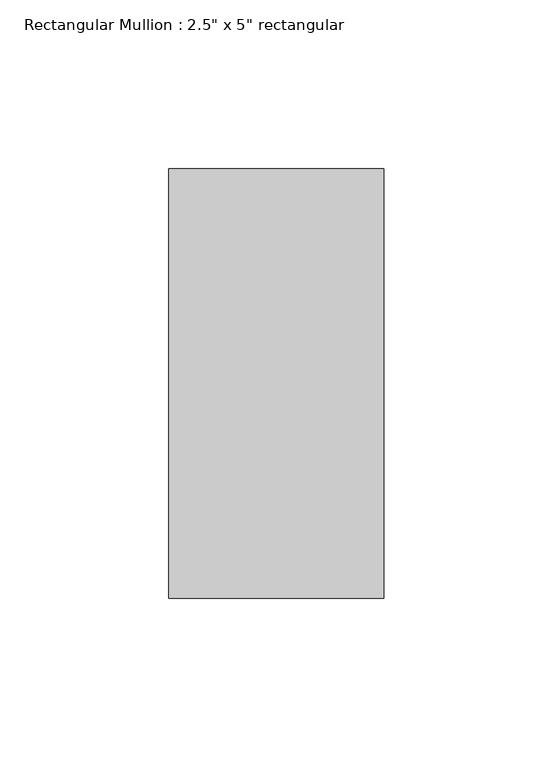
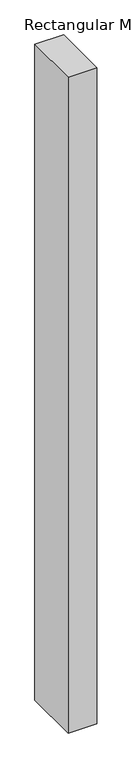
"""IFC4 building model written with IfcOpenShell, lengths in millimetres: member geometry."""

from ifc_helpers import new_model, si_unit, frame, origin, place, context, project, spatial, polyline, outline, extrude, source, transform, mapped, element, save


def member_bc6c8480(model_context):
    return source(origin(), model_context, "Body", "SweptSolid", [
        extrude(outline(polyline([(0.0, 63.5), (0.0, -63.5), (-63.5, -63.5), (-63.5, 63.5), (0.0, 63.5)])), frame((0.0, 0.0, -1536.2264761), z_axis=(0.0, 0.0, 1.0), x_axis=(1.0, 0.0, 0.0)), (0.0, 0.0, 1.0), 1536.2264761),
    ])


if __name__ == "__main__":
    model = new_model("IFC4")
    model_context = context("Model", 3, world=origin())
    ifc_project = project(units=[si_unit("LENGTHUNIT", "METRE", prefix="MILLI")], contexts=[model_context])
    site = spatial("IfcSite", under=ifc_project)
    building = spatial("IfcBuilding", under=site)
    placement = place(None, origin())
    member_shape = member_bc6c8480(model_context)
    element("IfcMember", 1, ObjectType="Rectangular Mullion : 2.5\" x 5\" rectangular", at=placement, inside=building, context=model_context, shape_type="MappedRepresentation", body=[
        mapped(member_shape, transform((0.0, 0.0, 0.0), x_axis=(1.0, 0.0, 0.0), y_axis=(0.0, 1.0, 0.0), z_axis=(0.0, 0.0, 1.0))),
    ])
    save(model, "model.ifc")

# Revit data of these elements
# Type "Rectangular Mullion : 2.5\" x 5\" rectangular"
#   built-in parameter 1007304 = 0.416667 (stored number, unit not read)
#   built-in parameter 1007301 = 0.104167 (stored number, unit not read)
#   built-in parameter 1007300 = 0.104167 (stored number, unit not read)
# Element 1 (IfcMember, "Rectangular Mullion : 2.5\" x 5\" rectangular")
#   Materials on its faces: "Aluminum"
# Materials
#   "Aluminum": class "Metal", colour RGB 247 247 247, transparency 0, Description = "Aluminum 6061", Cost = 0
